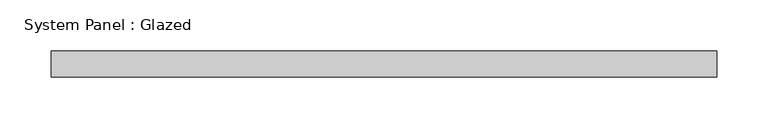
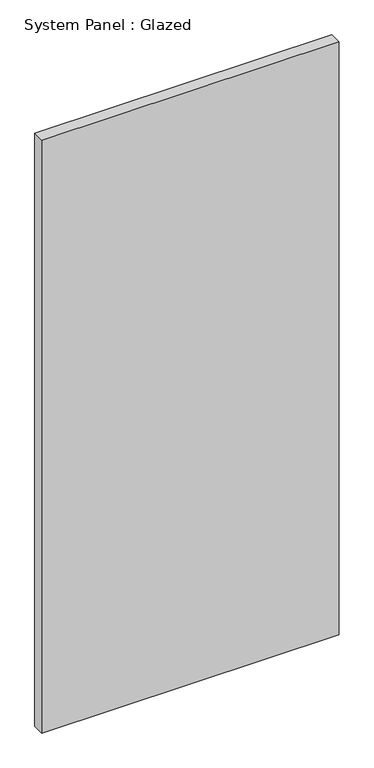
"""IFC4 building model written with IfcOpenShell, lengths in millimetres: plate geometry, System Panel : Glazed."""

from ifc_helpers import new_model, si_unit, origin, origin_with_axes, place, context, project, spatial, polyline, outline, extrude, source, transform, mapped, element, save


def system_panel_glazed_bf013b5c(model_context):
    return source(origin(), model_context, "Body", "SweptSolid", [
        extrude(outline(polyline([(323.85, 19.05), (-323.85, 19.05), (-323.85, 44.45), (323.85, 44.45), (323.85, 19.05)])), origin_with_axes(), (0.0, 0.0, 1.0), 1364.6991558),
    ])


if __name__ == "__main__":
    model = new_model("IFC4")
    model_context = context("Model", 3, world=origin())
    ifc_project = project(units=[si_unit("LENGTHUNIT", "METRE", prefix="MILLI")], contexts=[model_context])
    site = spatial("IfcSite", under=ifc_project)
    building = spatial("IfcBuilding", under=site)
    placement = place(None, origin())
    system_panel_glazed_shape = system_panel_glazed_bf013b5c(model_context)
    element("IfcPlate", 1, ObjectType="System Panel : Glazed", at=placement, inside=building, context=model_context, shape_type="MappedRepresentation", body=[
        mapped(system_panel_glazed_shape, transform((0.0, 0.0, 0.0), x_axis=(1.0, 0.0, 0.0), y_axis=(0.0, 1.0, 0.0), z_axis=(0.0, 0.0, 1.0))),
    ])
    save(model, "model.ifc")

# Revit data of these elements
# Type "System Panel : Glazed"
#   Construction Type Id = "GSP4R"
#   Analytic Construction = "1/8 in Pilkington single glazing"
#   Visual Light Transmittance = 0.9
#   Solar Heat Gain Coefficient = 0.86
#   Heat Transfer Coefficient (U) = 1.18115 BTU/(h·ft²·°F)
#   Define Thermal Properties by = 1
# Element 1 (IfcPlate, "System Panel : Glazed")
#   Materials on its faces: "Glass"
# Materials
#   "Glass": class "Glass", colour RGB 0 128 192, transparency 0.75, Description = "Soda Lime Glass", Cost = 0
